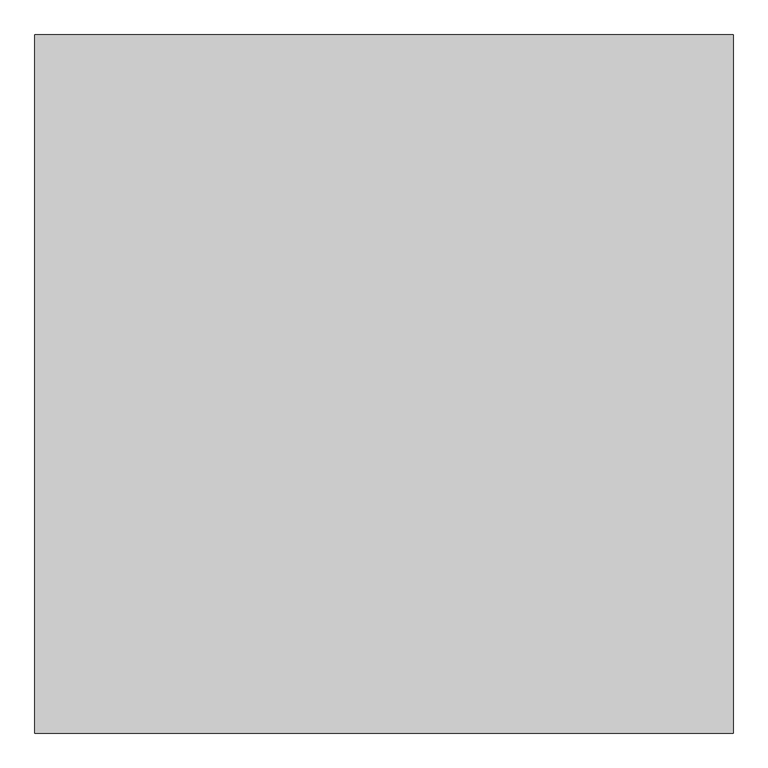
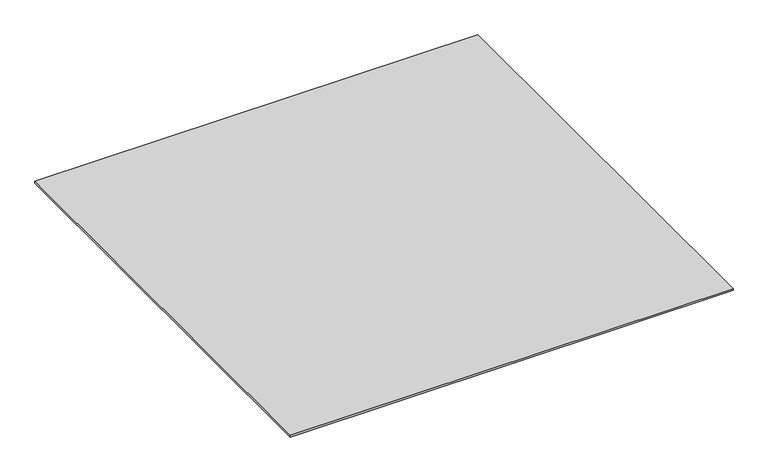
"""IFC4 building model written with IfcOpenShell, lengths in millimetres: furniture geometry."""

from ifc_helpers import new_model, si_unit, origin, origin_with_axes, place, context, project, spatial, polyline, outline, extrude, source, transform, mapped, element, save


def furniture_48082557(model_context):
    return source(origin(), model_context, "Body", "SweptSolid", [
        extrude(outline(polyline([(1250.0, 1250.0), (1250.0, -1250.0), (-1250.0, -1250.0), (-1250.0, 1250.0), (1250.0, 1250.0)])), origin_with_axes(), (0.0, 0.0, 1.0), 10.0),
    ])


if __name__ == "__main__":
    model = new_model("IFC4")
    model_context = context("Model", 3, world=origin())
    ifc_project = project(units=[si_unit("LENGTHUNIT", "METRE", prefix="MILLI")], contexts=[model_context])
    site = spatial("IfcSite", under=ifc_project)
    building = spatial("IfcBuilding", under=site)
    placement = place(None, origin())
    furniture_shape = furniture_48082557(model_context)
    element("IfcFurniture", 1, at=placement, inside=building, context=model_context, shape_type="MappedRepresentation", body=[
        mapped(furniture_shape, transform((0.0, 0.0, 0.0), x_axis=(1.0, 0.0, 0.0), y_axis=(0.0, 1.0, 0.0), z_axis=(0.0, 0.0, 1.0))),
    ])
    save(model, "model.ifc")

# Revit data of these elements
# Type
#   Width - Anchura = 2500 mm
#   Thickness - Espesor = 10 mm
#   Large - Largo = 2500 mm
#   Default Elevation = 1219.2 mm
